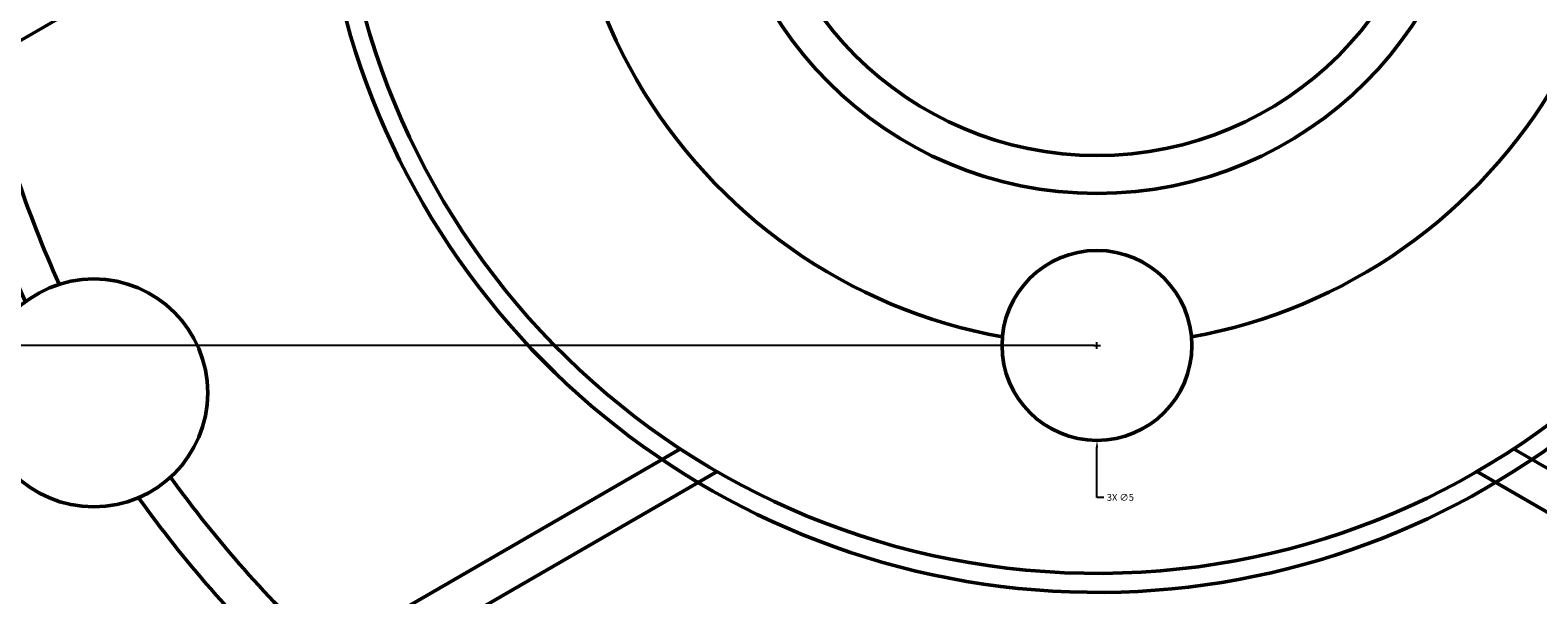
# Model space of a CAD drawing. Units: inches. Extents: x -19.9 to 72.3, y -39.8 to 57.5.
# Tile 3 of 8: x 0 to 39.7, y -7.2 to 7.6. Entities that reach past the tile are written whole.
import ezdxf

# ---------------------------------------------------------------- set-up
doc = ezdxf.new("R2010")
doc.units = ezdxf.units.IN
doc.header["$MEASUREMENT"] = 0
for name, color, linetype, lineweight in [('M-DIMS', 2, 'Continuous', 18), ('M-OUTL', 7, 'Continuous', 50), ('M-OUTL-HOLE', 7, 'Continuous', 50), ('M-OUTL-SLOT', 7, 'Continuous', 50)]:
    doc.layers.add(name, color=color, linetype=linetype, lineweight=lineweight)
doc.styles.get("Standard").update_dxf_attribs({"font": 'arial.ttf'})
doc.dimstyles.get("Standard").update_dxf_attribs({"dimtxt": 0.18, "dimasz": 0.18, "dimexe": 0.18, "dimexo": 0.0625, "dimgap": 0.09, "dimtad": 0, "dimtih": 1, "dimtoh": 1, "dimdec": 4, "dimzin": 0, "dimdsep": 46, "dimtxsty": 'Standard', "dimcen": 0.09, "dimadec": 0, "dimazin": 0, "dimtfac": 1, "dimtdec": 4, "dimtofl": 0, "dimtmove": 0, "dimatfit": 3, "dimfxl": 1, "dimtolj": 1, "dimtzin": 0, "dimarcsym": 0})

# ---------------------------------------------------------------- blocks, each defined once
blk = doc.blocks.new('FLANGE-MOUNT-D8-RELIEVED')
blk.add_circle((0, 0), 4)
for centre, radius, start, end in [((26.414, -15.25), 30, 109.4712, 138.6562), ((0, 0), 6, 250.4286, 49.5714), ((26.414, -15.25), 30, 161.3438, 190.5288)]:
    blk.add_arc(centre, radius, start, end)
blk = doc.blocks.new('FLANGE-HOLE-D6')
blk.add_circle((0, 0), 3)
blk = doc.blocks.new('HUB-HOLE-D5')
blk.add_circle((0, 0), 2.5)
blk = doc.blocks.new('FLANGE-STRAIGHT-SLOT')
for p, q in [((0, 0), (0, 21.114)), ((1, -0.54), (1, 20.869))]:
    blk.add_line(p, q)
blk = doc.blocks.new('FLANGE-INTERRUPTED-ARC-SLOT')
for radius, start, end in [(30, 192.5424, 204.3948), (31, 193.1227, 204.486), (30, 215.6052, 227.4576), (31, 215.514, 226.8773)]:
    blk.add_arc((26.414, 15.25), radius, start, end)
blk = doc.blocks.new('*D6')
at = {"layer": 'Defpoints', "color": 0, "transparency": 16777216}
for p in [(28.06, 43.841), (28.06, -17.159), (72.086, -17.159)]:
    blk.add_point(p, dxfattribs=at)
at = {"layer": 'M-DIMS', "color": 0, "lineweight": -2, "transparency": 16777216}
for p, q in [((28.122, 43.841), (72.266, 43.841)), ((72.086, 43.661), (72.086, 13.523)), ((72.086, -16.979), (72.086, 13.159)), ((28.122, -17.159), (72.266, -17.159))]:
    blk.add_line(p, q, dxfattribs=at)
at = {"layer": 'M-DIMS', "color": 0, "transparency": 16777216}
for points in [[(72.056, 43.661), (72.116, 43.661), (72.086, 43.841)], [(72.056, -16.979), (72.116, -16.979), (72.086, -17.159)]]:
    blk.add_solid(points, dxfattribs=at)
at = {"layer": 'M-DIMS', "color": 0, "transparency": 16777216, "insert": (72.086, 13.341), "char_height": 0.18, "attachment_point": 5}
blk.add_mtext('\\A1;61', dxfattribs=at)
blk = doc.blocks.new('*D9')
at = {"layer": 'Defpoints', "color": 0, "transparency": 16777216}
for p in [(15.936, 20.341), (-15.966, -0.659), (28.06, -0.659)]:
    blk.add_point(p, dxfattribs=at)
at = {"layer": 'M-DIMS', "color": 0, "lineweight": -2, "transparency": 16777216}
for p, q in [((15.873, 20.341), (-16.146, 20.341)), ((-15.966, 20.161), (-15.966, 10.022)), ((-15.966, -0.479), (-15.966, 9.661)), ((27.997, -0.659), (-16.146, -0.659))]:
    blk.add_line(p, q, dxfattribs=at)
at = {"layer": 'M-DIMS', "color": 0, "transparency": 16777216}
for points in [[(-15.996, 20.161), (-15.936, 20.161), (-15.966, 20.341)], [(-15.996, -0.479), (-15.936, -0.479), (-15.966, -0.659)]]:
    blk.add_solid(points, dxfattribs=at)
at = {"layer": 'M-DIMS', "color": 0, "transparency": 16777216, "insert": (-15.966, 9.841), "char_height": 0.18, "attachment_point": 5}
blk.add_mtext('\\A1;21', dxfattribs=at)
blk = doc.blocks.new('*D11')
at = {"layer": 'Defpoints', "color": 0, "transparency": 16777216}
for p in [(5.703, 46.51), (50.417, -19.828)]:
    blk.add_point(p, dxfattribs=at)
at = {"layer": 'M-DIMS', "color": 0, "lineweight": -2, "transparency": 16777216}
for p, q in [((27.97, 13.341), (28.15, 13.341)), ((28.06, 13.251), (28.06, 13.431)), ((63.831, -39.729), (50.517, -19.977)), ((64.011, -39.729), (63.831, -39.729))]:
    blk.add_line(p, q, dxfattribs=at)
at = {"layer": 'M-DIMS', "color": 0, "transparency": 16777216}
blk.add_solid([(50.542, -19.96), (50.492, -19.994), (50.417, -19.828)], dxfattribs=at)
at = {"layer": 'M-DIMS', "color": 0, "transparency": 16777216, "insert": (64.327, -39.729), "char_height": 0.18, "attachment_point": 5}
blk.add_mtext('\\A1;∅80', dxfattribs=at)
blk = doc.blocks.new('*D12')
at = {"layer": 'Defpoints', "color": 0, "transparency": 16777216}
for p in [(28.06, 13.341), (-1.285, 3.349)]:
    blk.add_point(p, dxfattribs=at)
at = {"layer": 'M-DIMS', "color": 0, "lineweight": -2, "transparency": 16777216}
for p, q in [((27.97, 13.341), (28.15, 13.341)), ((28.06, 13.251), (28.06, 13.431)), ((-18.893, -2.647), (-1.456, 3.291)), ((-19.073, -2.647), (-18.893, -2.647))]:
    blk.add_line(p, q, dxfattribs=at)
at = {"layer": 'M-DIMS', "color": 0, "transparency": 16777216}
blk.add_solid([(-1.466, 3.319), (-1.446, 3.262), (-1.285, 3.349)], dxfattribs=at)
at = {"layer": 'M-DIMS', "color": 0, "transparency": 16777216, "insert": (-19.557, -2.647), "char_height": 0.18, "attachment_point": 5}
blk.add_mtext('\\A1;4X R31', dxfattribs=at)
blk = doc.blocks.new('*D22')
at = {"layer": 'Defpoints', "color": 0, "transparency": 16777216}
for p in [(28.06, 1.841), (28.06, -3.159)]:
    blk.add_point(p, dxfattribs=at)
at = {"layer": 'M-DIMS', "color": 0, "lineweight": -2, "transparency": 16777216}
for p, q in [((27.97, -0.659), (28.15, -0.659)), ((28.06, -0.749), (28.06, -0.569)), ((28.06, -4.659), (28.06, -3.339)), ((28.24, -4.659), (28.06, -4.659))]:
    blk.add_line(p, q, dxfattribs=at)
at = {"layer": 'M-DIMS', "color": 0, "transparency": 16777216}
blk.add_solid([(28.09, -3.339), (28.03, -3.339), (28.06, -3.159)], dxfattribs=at)
at = {"layer": 'M-DIMS', "color": 0, "transparency": 16777216, "insert": (28.676, -4.659), "char_height": 0.18, "attachment_point": 5}
blk.add_mtext('\\A1;3X ∅5', dxfattribs=at)

msp = doc.modelspace()

# ---------------------------------------------------------------- linework, layer by layer
at = {"layer": 'M-OUTL'}
for radius in [40, 10, 9]:
    msp.add_circle((28.06, 13.341), radius, dxfattribs=at)
for radius, start, end in [(20, 0, 356.7437), (20.5, 183.9584, 60.8036), (14, 160.245, 259.755), (14, 280.245, 19.755)]:
    msp.add_arc((28.06, 13.341), radius, start, end, dxfattribs=at)

# ---------------------------------------------------------------- block references
at = {"layer": 'M-OUTL-HOLE', "rotation": 120}
msp.add_blockref('FLANGE-MOUNT-D8-RELIEVED', (28.06, -17.159), dxfattribs=at)
at = {"layer": 'M-OUTL-HOLE'}
for name, p in [('HUB-HOLE-D5', (28.06, -0.659)), ('FLANGE-HOLE-D6', (1.646, -1.909))]:
    msp.add_blockref(name, p, dxfattribs=at)
at = {"layer": 'M-OUTL-SLOT'}
for p, rotation in [((8.092, 12.205), 119.9999999999999), ((39.028, -3.383), 240)]:
    msp.add_blockref('FLANGE-STRAIGHT-SLOT', p, dxfattribs=dict(at, rotation=rotation))
msp.add_blockref('FLANGE-INTERRUPTED-ARC-SLOT', (1.646, -1.909), dxfattribs=at)
at = {"layer": 'M-OUTL-SLOT', "extrusion": (0, 0, -1), "zscale": -1, "rotation": 239.9999999999999}
msp.add_blockref('FLANGE-STRAIGHT-SLOT', (-17.092, -3.383), dxfattribs=at)

# ---------------------------------------------------------------- dimensions: what is measured, and where the dimension line sits
at = {"layer": 'M-DIMS'}
dim = msp.add_diameter_dim_2p(p1=(5.703, 46.51), p2=(50.417, -19.828), dimstyle='Standard', override={"dimdec": 0, "dimlfac": 1, "dimrnd": 0, "dimzin": 0, "dimdsep": 46, "dimlunit": 2}, dxfattribs=at)
dim.commit()
dim.dimension.update_dxf_attribs({"geometry": '*D11', "text_midpoint": (64.327, -39.729), "dimtype": 163})
for base, p1, p2, picture, middle in [((72.086, -17.159), (28.06, 43.841), (28.06, -17.159), '*D6', (72.086, 13.341)), ((-15.966, -0.659), (15.936, 20.341), (28.06, -0.659), '*D9', (-15.966, 9.841))]:
    dim = msp.add_linear_dim(base=base, p1=p1, p2=p2, angle=90, dimstyle='Standard', override={"dimdec": 0, "dimlfac": 1, "dimrnd": 0, "dimzin": 0, "dimdsep": 46, "dimlunit": 2}, dxfattribs=at)
    dim.commit()
    dim.dimension.update_dxf_attribs({"geometry": picture, "text_midpoint": middle})
dim = msp.add_radius_dim(center=(28.06, 13.341), mpoint=(-1.285, 3.349), text='4X <>', dimstyle='Standard', override={"dimdec": 0, "dimlfac": 1, "dimrnd": 0, "dimzin": 0, "dimdsep": 46, "dimlunit": 2}, dxfattribs=at)
dim.commit()
dim.dimension.update_dxf_attribs({"geometry": '*D12', "text_midpoint": (-19.557, -2.647), "dimtype": 164})
dim = msp.add_diameter_dim_2p(p1=(28.06, 1.841), p2=(28.06, -3.159), text='3X <>', dimstyle='Standard', override={"dimdec": 0, "dimlfac": 1, "dimrnd": 0, "dimzin": 0, "dimdsep": 46, "dimlunit": 2}, dxfattribs=at)
dim.commit()
dim.dimension.update_dxf_attribs({"geometry": '*D22', "text_midpoint": (28.676, -4.659), "dimtype": 163})

doc.saveas('drawing.dxf')
